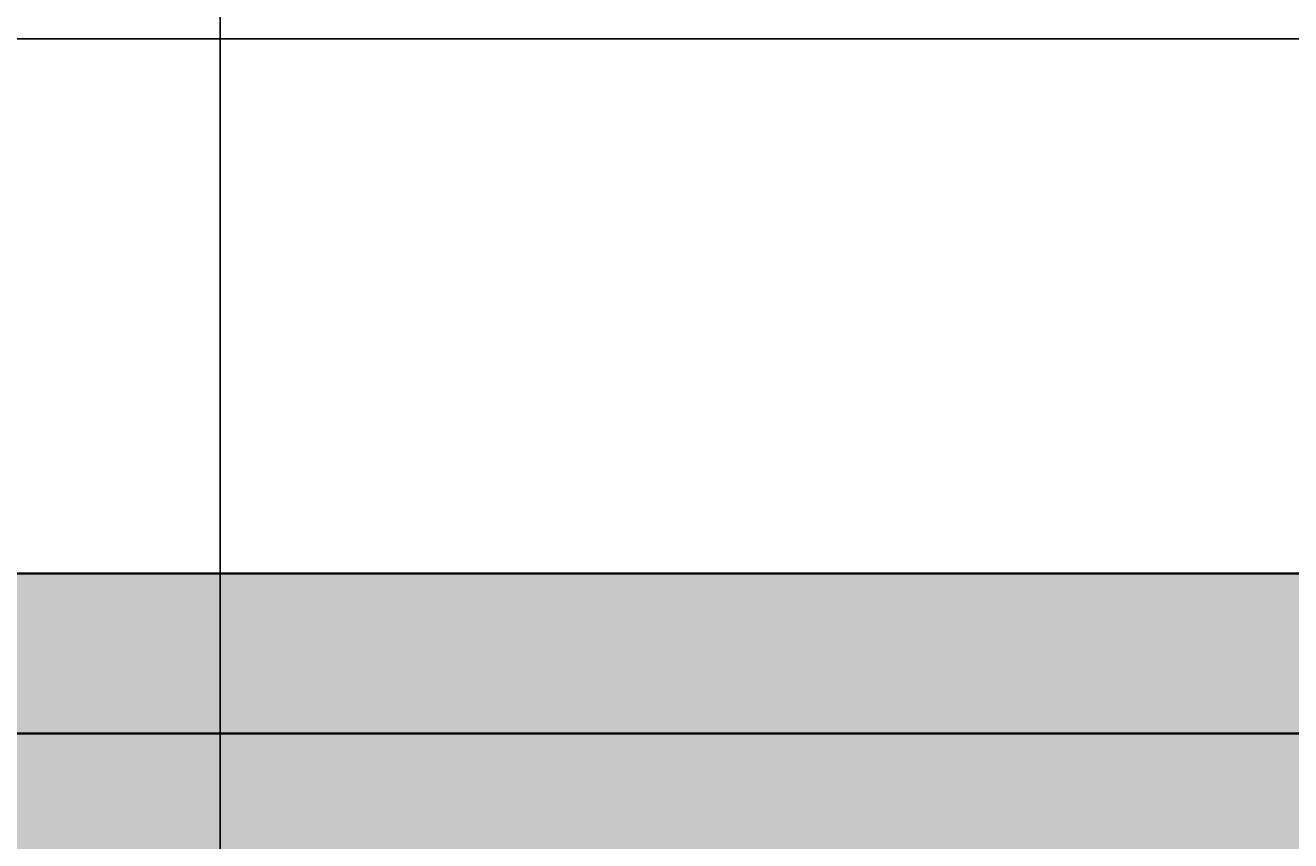
# Model space of a CAD drawing. Units: feet. Extents: x 2695 to 2912, y 795 to 1139.
# Tile 73 of 83: x 2805 to 2840, y 1100 to 1123. Entities that reach past the tile are written whole.
import ezdxf

# ---------------------------------------------------------------- set-up
doc = ezdxf.new("R2010")
doc.units = ezdxf.units.FT
for name, color, linetype, lineweight in [('A-ANNO-DIMS', 2, 'Continuous', 18), ('A-ELEV', 7, 'Continuous', 35), ('A-ELEV-PATT', 252, 'Continuous', 13)]:
    doc.layers.add(name, color=color, linetype=linetype, lineweight=lineweight)
doc.styles.get("Standard").update_dxf_attribs({"font": 'arial.ttf'})
doc.dimstyles.get("Standard").update_dxf_attribs({"dimtxt": 0.18, "dimasz": 0.18, "dimexe": 0.18, "dimexo": 0.0625, "dimgap": 0.09, "dimtad": 0, "dimtih": 1, "dimtoh": 1, "dimdec": 1, "dimzin": 0, "dimdsep": 46, "dimlunit": 3, "dimtxsty": 'Standard', "dimcen": 0.09, "dimadec": 0, "dimazin": 0, "dimtfac": 1, "dimtdec": 1, "dimtofl": 0, "dimtmove": 0, "dimatfit": 3, "dimfxl": 1, "dimtolj": 1, "dimtzin": 0, "dimarcsym": 0})

# ---------------------------------------------------------------- blocks, each defined once
blk = doc.blocks.new('*D10')
at = {"layer": 'A-ANNO-DIMS', "color": 0, "lineweight": -2, "transparency": 16777216}
for p, q in [((2778.034, 1020.886), (2778.034, 1138.886)), ((2778.214, 1138.706), (2810.411, 1138.706)), ((2843.395, 1138.706), (2811.198, 1138.706)), ((2843.575, 1020.886), (2843.575, 1138.886))]:
    blk.add_line(p, q, dxfattribs=at)
at = {"layer": 'A-ANNO-DIMS', "color": 0, "transparency": 16777216}
for points in [[(2778.214, 1138.736), (2778.214, 1138.676), (2778.034, 1138.706)], [(2843.395, 1138.736), (2843.395, 1138.676), (2843.575, 1138.706)]]:
    blk.add_solid(points, dxfattribs=at)
at = {"layer": 'Defpoints', "color": 0, "transparency": 16777216}
for p in [(2843.575, 1138.706), (2778.034, 1020.824), (2843.575, 1020.824)]:
    blk.add_point(p, dxfattribs=at)
at = {"layer": 'A-ANNO-DIMS', "color": 0, "transparency": 16777216, "insert": (2810.805, 1138.706), "char_height": 0.18, "attachment_point": 5}
blk.add_mtext('\\A1;65.54', dxfattribs=at)
blk = doc.blocks.new('*D22')
at = {"layer": 'A-ANNO-DIMS', "color": 0, "lineweight": -2, "transparency": 16777216}
for p, q in [((2770.699, 1122.931), (2911.424, 1122.931)), ((2911.244, 1122.751), (2911.244, 1115.565)), ((2911.244, 1108.015), (2911.244, 1115.201)), ((2895.532, 1107.835), (2911.424, 1107.835))]:
    blk.add_line(p, q, dxfattribs=at)
at = {"layer": 'A-ANNO-DIMS', "color": 0, "transparency": 16777216}
for points in [[(2911.214, 1122.751), (2911.274, 1122.751), (2911.244, 1122.931)], [(2911.214, 1108.015), (2911.274, 1108.015), (2911.244, 1107.835)]]:
    blk.add_solid(points, dxfattribs=at)
at = {"layer": 'Defpoints', "color": 0, "transparency": 16777216}
for p in [(2770.636, 1122.931), (2911.244, 1122.931), (2895.469, 1107.835)]:
    blk.add_point(p, dxfattribs=at)
at = {"layer": 'A-ANNO-DIMS', "color": 0, "transparency": 16777216, "insert": (2911.244, 1115.383), "char_height": 0.18, "attachment_point": 5}
blk.add_mtext('\\A1;15.095', dxfattribs=at)
blk = doc.blocks.new('*D49')
at = {"layer": 'A-ANNO-DIMS', "color": 0, "lineweight": -2, "transparency": 16777216}
for p, q in [((2772.522, 972.03), (2772.522, 1138.886)), ((2772.702, 1138.706), (2790.888, 1138.706)), ((2809.861, 1138.706), (2791.674, 1138.706)), ((2810.041, 972.03), (2810.041, 1138.886))]:
    blk.add_line(p, q, dxfattribs=at)
at = {"layer": 'A-ANNO-DIMS', "color": 0, "transparency": 16777216}
for points in [[(2772.702, 1138.736), (2772.702, 1138.676), (2772.522, 1138.706)], [(2809.861, 1138.736), (2809.861, 1138.676), (2810.041, 1138.706)]]:
    blk.add_solid(points, dxfattribs=at)
at = {"layer": 'Defpoints', "color": 0, "transparency": 16777216}
for p in [(2810.041, 1138.706), (2772.522, 971.967), (2810.041, 971.967)]:
    blk.add_point(p, dxfattribs=at)
at = {"layer": 'A-ANNO-DIMS', "color": 0, "transparency": 16777216, "insert": (2791.281, 1138.706), "char_height": 0.18, "attachment_point": 5}
blk.add_mtext('\\A1;37.52', dxfattribs=at)
blk = doc.blocks.new('*D50')
at = {"layer": 'A-ANNO-DIMS', "color": 0, "lineweight": -2, "transparency": 16777216}
for p, q in [((2810.041, 972.03), (2810.041, 1138.886)), ((2810.221, 1138.706), (2848.721, 1138.706)), ((2888.008, 1138.706), (2849.508, 1138.706)), ((2888.188, 972.03), (2888.188, 1138.886))]:
    blk.add_line(p, q, dxfattribs=at)
at = {"layer": 'A-ANNO-DIMS', "color": 0, "transparency": 16777216}
for points in [[(2810.221, 1138.736), (2810.221, 1138.676), (2810.041, 1138.706)], [(2888.008, 1138.736), (2888.008, 1138.676), (2888.188, 1138.706)]]:
    blk.add_solid(points, dxfattribs=at)
at = {"layer": 'Defpoints', "color": 0, "transparency": 16777216}
for p in [(2888.188, 1138.706), (2810.041, 971.967), (2888.188, 971.967)]:
    blk.add_point(p, dxfattribs=at)
at = {"layer": 'A-ANNO-DIMS', "color": 0, "transparency": 16777216, "insert": (2849.114, 1138.706), "char_height": 0.18, "attachment_point": 5}
blk.add_mtext('\\A1;78.15', dxfattribs=at)

msp = doc.modelspace()

# ---------------------------------------------------------------- hatches: boundary and pattern name
at = {"layer": 'A-ELEV-PATT'}
h = msp.add_hatch(color=256, dxfattribs=at)
h.set_gradient(color1=(255, 255, 255), tint=1)
h.paths.add_polyline_path([(2770.6361, 1122.9306), (2710.6361, 1122.9306), (2710.6361, 1118.4096), (2770.6361, 1118.4096)])
h.paths.add_polyline_path([(2890.6361, 1107.8588), (2770.6361, 1107.8588), (2770.6361, 1103.3378), (2890.6361, 1103.3378)])
h.paths.add_polyline_path([(2890.6361, 1062.9306), (2710.6361, 1062.9306), (2710.6361, 1056.9306), (2710.6361, 936.9306), (2710.6361, 924.3105), (2716.5358, 924.3105), (2890.6361, 924.3105), (2890.6361, 936.9306), (2715.8852, 936.9306), (2715.8852, 1050.3105), (2890.6361, 1050.3105)])
h.paths.add_polyline_path([(2716.5358, 924.3105), (2710.6361, 924.3105), (2710.6361, 810.9306), (2716.5358, 810.9306)])
h = msp.add_hatch(color=256, dxfattribs=at)
h.set_gradient(color1=(147, 149, 152), color2=(147, 149, 152), tint=1)
h.paths.add_polyline_path([(2770.6361, 1118.4096), (2710.6361, 1118.4096), (2710.6361, 1062.9306), (2770.6361, 1062.9306)])
h.paths.add_polyline_path([(2890.6361, 1103.3378), (2770.6361, 1103.3378), (2770.6361, 1062.9306), (2890.6361, 1062.9306)])
h.paths.add_polyline_path([(2730.7081, 1048.1052), (2755.1125, 1048.1052), (2755.1125, 936.9306), (2770.6361, 936.9306), (2770.6361, 1050.3105), (2715.8852, 1050.3105), (2715.8852, 936.9306), (2730.7081, 936.9306)])
h.paths.add_polyline_path([(2890.6361, 1050.3105), (2770.6361, 1050.3105), (2770.6361, 971.9673), (2778.0341, 971.9673), (2778.0341, 1020.8235), (2843.575, 1020.8235), (2843.575, 971.9673), (2890.6361, 971.9673)])
h.paths.add_polyline_path([(2888.1882, 970.7156), (2843.575, 970.7156), (2843.575, 964.8267), (2888.1882, 964.8267)])
h.paths.add_polyline_path([(2888.1882, 964.1328), (2843.575, 964.1328), (2843.575, 956.614), (2888.1882, 956.614)])
h.paths.add_polyline_path([(2888.1882, 955.9202), (2843.575, 955.9202), (2843.575, 949.2892), (2888.1882, 949.2892)])
h.paths.add_polyline_path([(2888.1882, 948.5954), (2843.575, 948.5954), (2843.575, 941.3507), (2888.1882, 941.3507)])
h.paths.add_polyline_path([(2888.1882, 940.6569), (2843.575, 940.6569), (2843.575, 936.9306), (2888.1882, 936.9306)])
h.paths.add_polyline_path([(2890.6361, 970.7156), (2888.9368, 970.7156), (2888.9368, 964.8267), (2890.6361, 964.8267)])
h.paths.add_polyline_path([(2890.6361, 964.1328), (2888.9368, 964.1328), (2888.9368, 956.614), (2890.6361, 956.614)])
h.paths.add_polyline_path([(2890.6361, 955.9202), (2888.9368, 955.9202), (2888.9368, 949.2892), (2890.6361, 949.2892)])
h.paths.add_polyline_path([(2890.6361, 940.6569), (2888.9368, 940.6569), (2888.9368, 936.9306), (2890.6361, 936.9306)])
h.paths.add_polyline_path([(2890.6361, 948.5954), (2888.9368, 948.5954), (2888.9368, 941.3507), (2890.6361, 941.3507)])
h.paths.add_polyline_path([(2772.5216, 970.7156), (2770.6361, 970.7156), (2770.6361, 964.8267), (2772.5216, 964.8267)])
h.paths.add_polyline_path([(2772.5216, 964.1328), (2770.6361, 964.1328), (2770.6361, 956.614), (2772.5216, 956.614)])
h.paths.add_polyline_path([(2772.5216, 955.9202), (2770.6361, 955.9202), (2770.6361, 949.2892), (2772.5216, 949.2892)])
h.paths.add_polyline_path([(2772.5216, 948.5954), (2770.6361, 948.5954), (2770.6361, 941.3507), (2772.5216, 941.3507)])
h.paths.add_polyline_path([(2772.5216, 940.6569), (2770.6361, 940.6569), (2770.6361, 936.9306), (2772.5216, 936.9306)])
h.paths.add_polyline_path([(2778.0341, 940.6569), (2773.2702, 940.6569), (2773.2702, 936.9306), (2778.0341, 936.9306)])
h.paths.add_polyline_path([(2778.0341, 970.7156), (2773.2702, 970.7156), (2773.2702, 964.8267), (2778.0341, 964.8267)])
h.paths.add_polyline_path([(2778.0341, 964.1328), (2773.2702, 964.1328), (2773.2702, 956.614), (2778.0341, 956.614)])
h.paths.add_polyline_path([(2778.0341, 955.9202), (2773.2702, 955.9202), (2773.2702, 949.2892), (2778.0341, 949.2892)])
h.paths.add_polyline_path([(2778.0341, 948.5954), (2773.2702, 948.5954), (2773.2702, 941.3507), (2778.0341, 941.3507)])
h.paths.add_polyline_path([(2810.0407, 940.6569), (2780.0341, 940.6569), (2780.0341, 936.9306), (2810.0407, 936.9306)])
h.paths.add_polyline_path([(2890.6361, 924.3105), (2770.6361, 924.3105), (2770.6361, 810.9306), (2773.5029, 810.9306), (2773.5029, 905.5143), (2805.9398, 905.5143), (2838.3767, 905.5143), (2838.3767, 810.9306), (2890.6361, 810.9306)])
h = msp.add_hatch(color=256, dxfattribs=at)
h.set_gradient(color1=(199, 200, 202), color2=(213, 227, 240), centered=1)
h.paths.add_polyline_path([(2890.6361, 1103.3378), (2770.6361, 1103.3378), (2770.6361, 1062.9306), (2890.6361, 1062.9306)])

# ---------------------------------------------------------------- linework, layer by layer
at = {"layer": 'A-ELEV'}
for p, q in [((2770.6361, 1107.8588), (2890.6361, 1107.8588)), ((2895.4694, 1107.8352), (2770.6361, 1107.8588)), ((2770.6361, 1103.3378), (2895.4694, 1103.3378))]:
    msp.add_line(p, q, dxfattribs=at)
msp.add_lwpolyline([(2770.6361, 1103.3378), (2890.6361, 1103.3378)], dxfattribs=at)

# ---------------------------------------------------------------- dimensions: what is measured, and where the dimension line sits
at = {"layer": 'A-ANNO-DIMS'}
for base, p1, p2, picture, middle in [((2810.0407, 1138.7056), (2772.5216, 971.9673), (2810.0407, 971.9673), '*D49', (2791.2811, 1138.7056)), ((2843.575, 1138.7056), (2778.0341, 1020.8235), (2843.575, 1020.8235), '*D10', (2810.8045, 1138.7056)), ((2888.1882, 1138.7056), (2810.0407, 971.9673), (2888.1882, 971.9673), '*D50', (2849.1144, 1138.7056))]:
    dim = msp.add_linear_dim(base=base, p1=p1, p2=p2, dimstyle='Standard', override={"dimdec": 2, "dimlfac": 1, "dimrnd": 0, "dimzin": 0, "dimdsep": 46, "dimlunit": 2}, dxfattribs=at)
    dim.commit()
    dim.dimension.update_dxf_attribs({"geometry": picture, "text_midpoint": middle})
dim = msp.add_linear_dim(base=(2911.2444, 1122.9306), p1=(2895.4694, 1107.8352), p2=(2770.6361, 1122.9306), angle=90, dimstyle='Standard', override={"dimdec": 3, "dimlfac": 1, "dimrnd": 0, "dimzin": 0, "dimdsep": 46, "dimlunit": 2}, dxfattribs=at)
dim.commit()
dim.dimension.update_dxf_attribs({"geometry": '*D22', "text_midpoint": (2911.2444, 1115.3829)})

doc.saveas('drawing.dxf')
